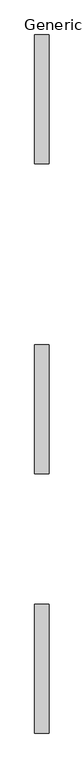
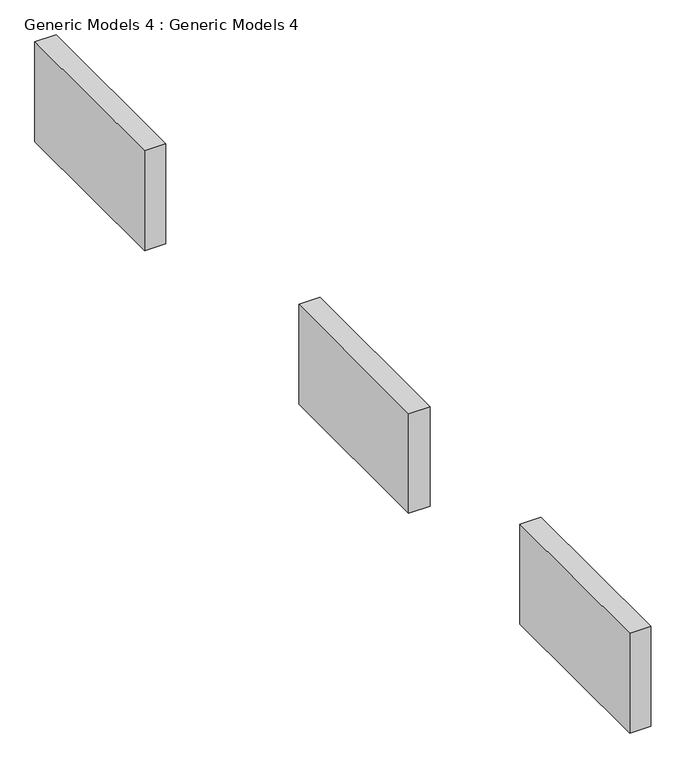
"""IFC4 building model written with IfcOpenShell, lengths in millimetres: proxy geometry, Generic Models 4 : Generic Models 4."""

from ifc_helpers import new_model, si_unit, frame, origin, place, context, project, spatial, polyline, outline, extrude, source, transform, mapped, element, save


def generic_models_4_generic_models_4_994ceaf2(model_context):
    return source(origin(), model_context, "Body", "SweptSolid", [
        extrude(outline(polyline([(-6115.6922047, 5197.9152598), (-6115.6922047, 7941.1152598), (-5810.8922047, 7941.1152598), (-5810.8922047, 5197.9152598), (-6115.6922047, 5197.9152598)])), frame((0.0, 0.0, 404.8717142), z_axis=(0.0, 0.0, 1.0), x_axis=(1.0, 0.0, 0.0)), (0.0, 0.0, 1.0), 1524.0),
        extrude(outline(polyline([(-6115.6922047, -1404.9064015), (-6115.6922047, 1338.2935985), (-5810.8922047, 1338.2935985), (-5810.8922047, -1404.9064015), (-6115.6922047, -1404.9064015)])), frame((0.0, 0.0, 404.8717142), z_axis=(0.0, 0.0, 1.0), x_axis=(1.0, 0.0, 0.0)), (0.0, 0.0, 1.0), 1524.0),
        extrude(outline(polyline([(-6115.6922047, -6929.4064015), (-6115.6922047, -4186.2064015), (-5810.8922047, -4186.2064015), (-5810.8922047, -6929.4064015), (-6115.6922047, -6929.4064015)])), frame((0.0, 0.0, 404.8717142), z_axis=(0.0, 0.0, 1.0), x_axis=(1.0, 0.0, 0.0)), (0.0, 0.0, 1.0), 1524.0),
    ])


if __name__ == "__main__":
    model = new_model("IFC4")
    model_context = context("Model", 3, world=origin())
    ifc_project = project(units=[si_unit("LENGTHUNIT", "METRE", prefix="MILLI")], contexts=[model_context])
    site = spatial("IfcSite", under=ifc_project)
    building = spatial("IfcBuilding", under=site)
    placement = place(None, origin())
    generic_models_4_generic_models_4_shape = generic_models_4_generic_models_4_994ceaf2(model_context)
    element("IfcBuildingElementProxy", 1, Name="Generic Models 4 : Generic Models 4", ObjectType="Generic Models 4 : Generic Models 4", at=placement, inside=building, context=model_context, shape_type="MappedRepresentation", body=[
        mapped(generic_models_4_generic_models_4_shape, transform((0.0, 0.0, 0.0), x_axis=(1.0, 0.0, 0.0), y_axis=(0.0, 1.0, 0.0), z_axis=(0.0, 0.0, 1.0))),
    ])
    save(model, "model.ifc")

# Revit data of these elements
# Element 1 (IfcBuildingElementProxy, "Generic Models 4 : Generic Models 4")
#   Materials on its faces: "Parking Stripe"
# Materials
#   "Parking Stripe": class "Paint", colour RGB 250 250 91, transparency 0, Cost = 0
